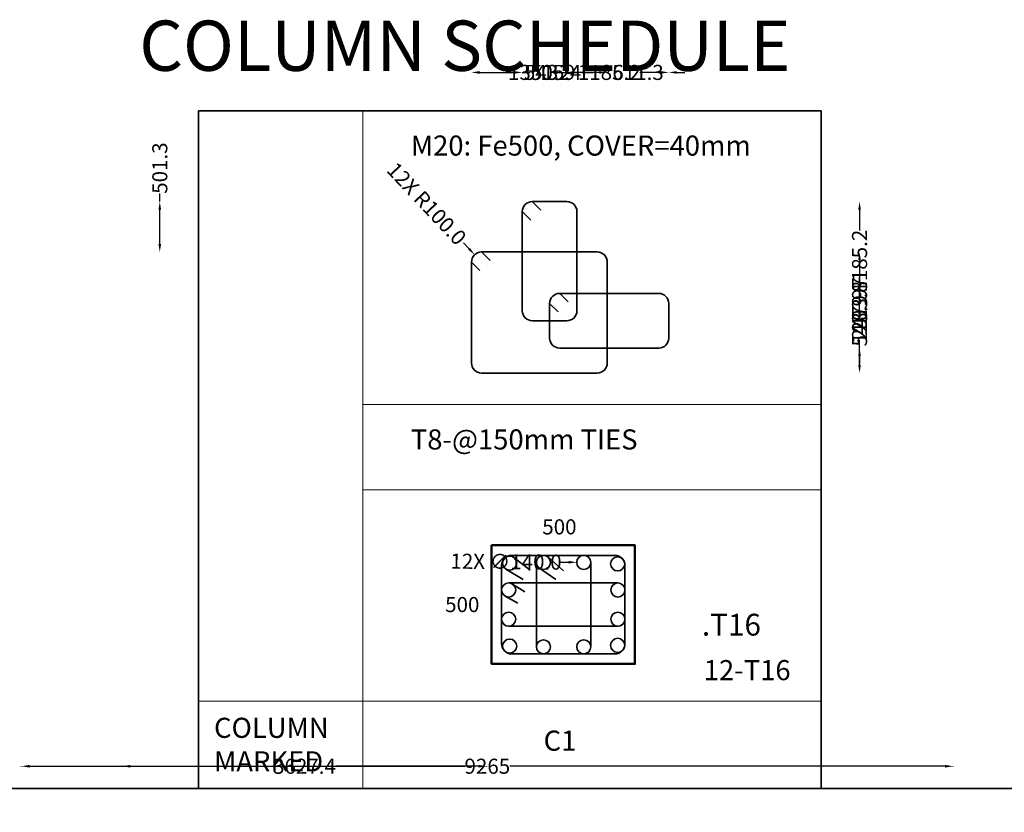
# Model space of a CAD drawing. Units: millimetres. Extents: x -19888 to 14444, y 67066 to 90098.
# Tile 6 of 7: x -7807 to 1986, y 82214 to 90098. Entities that reach past the tile are written whole.
import ezdxf

# ---------------------------------------------------------------- set-up
doc = ezdxf.new("R2010")
doc.units = ezdxf.units.MM
doc.header["$LTSCALE"] = 50
doc.header["$MEASUREMENT"] = 0
for name, color, linetype, lineweight in [('S-ANNO-DIMS', 2, 'Continuous', 18), ('S-ANNO-TABL', 7, 'Continuous', 18), ('S-ANNO-TEXT', 7, 'Continuous', 25), ('S-ANNO-TTLB', 7, 'Continuous', 35), ('S-COLS', 4, 'Continuous', 50), ('S-REIN', 6, 'Continuous', 35)]:
    doc.layers.add(name, color=color, linetype=linetype, lineweight=lineweight)
doc.styles.get("Standard").update_dxf_attribs({"font": 'arial.ttf'})
doc.dimstyles.get("Standard").update_dxf_attribs({"dimtxt": 150, "dimasz": 80, "dimexe": 0.18, "dimexo": 0.0625, "dimgap": 0.09, "dimtad": 0, "dimdec": 0, "dimzin": 0, "dimdsep": 46, "dimtxsty": 'Standard', "dimcen": 0.09, "dimadec": 0, "dimazin": 0, "dimtfac": 1, "dimtdec": 0, "dimtofl": 0, "dimtmove": 0, "dimatfit": 3, "dimfxl": 1, "dimfxlon": 1, "dimtolj": 1, "dimtzin": 0, "dimarcsym": 0})

# ---------------------------------------------------------------- blocks, each defined once
blk = doc.blocks.new('*D51')
at = {"layer": 'Defpoints', "color": 0, "ltscale": 50, "transparency": 16777216}
for p in [(1476.3, 82672.6), (-7788.5, 81596.7), (1476.3, 81596.7)]:
    blk.add_point(p, dxfattribs=at)
at = {"layer": 'S-ANNO-DIMS', "color": 0, "lineweight": -2, "ltscale": 50, "transparency": 16777216}
for p, q in [((-7788.5, 82671.6), (-7788.5, 82672.8)), ((-7708.5, 82672.6), (-3380.7, 82672.6)), ((1396.3, 82672.6), (-2931.5, 82672.6)), ((1476.3, 82671.6), (1476.3, 82672.8))]:
    blk.add_line(p, q, dxfattribs=at)
at = {"layer": 'S-ANNO-DIMS', "color": 0, "ltscale": 50, "transparency": 16777216}
for points in [[(-7708.5, 82686), (-7708.5, 82659.3), (-7788.5, 82672.6)], [(1396.3, 82686), (1396.3, 82659.3), (1476.3, 82672.6)]]:
    blk.add_solid(points, dxfattribs=at)
at = {"layer": 'S-ANNO-DIMS', "color": 0, "ltscale": 50, "transparency": 16777216, "insert": (-3156.1, 82672.6), "char_height": 150, "attachment_point": 5}
blk.add_mtext('\\A1;9265', dxfattribs=at)
blk = doc.blocks.new('*D57')
at = {"layer": 'Defpoints', "color": 0, "ltscale": 50, "transparency": 16777216}
for p in [(-3161.2, 82672.6), (-6788.5, 80274.3), (-3161.2, 80215.4)]:
    blk.add_point(p, dxfattribs=at)
at = {"layer": 'S-ANNO-DIMS', "color": 0, "lineweight": -2, "ltscale": 50, "transparency": 16777216}
for p, q in [((-6788.5, 82671.6), (-6788.5, 82672.8)), ((-6708.5, 82672.6), (-5286, 82672.6)), ((-3241.2, 82672.6), (-4663.8, 82672.6)), ((-3161.2, 82671.6), (-3161.2, 82672.8))]:
    blk.add_line(p, q, dxfattribs=at)
at = {"layer": 'S-ANNO-DIMS', "color": 0, "ltscale": 50, "transparency": 16777216}
for points in [[(-6708.5, 82686), (-6708.5, 82659.3), (-6788.5, 82672.6)], [(-3241.2, 82686), (-3241.2, 82659.3), (-3161.2, 82672.6)]]:
    blk.add_solid(points, dxfattribs=at)
at = {"layer": 'S-ANNO-DIMS', "color": 0, "ltscale": 50, "transparency": 16777216, "insert": (-4974.9, 82672.6), "char_height": 150, "attachment_point": 5}
blk.add_mtext('\\A1;3627.4', dxfattribs=at)
blk = doc.blocks.new('*D80')
at = {"layer": 'Defpoints', "color": 0, "ltscale": 50, "transparency": 16777216}
for p in [(-1962.8, 89573.9), (-3314, 86683.8), (-1962.8, 86683.8)]:
    blk.add_point(p, dxfattribs=at)
at = {"layer": 'S-ANNO-DIMS', "color": 0, "lineweight": -2, "ltscale": 50, "transparency": 16777216}
for p, q in [((-3314, 89572.9), (-3314, 89574.1)), ((-3234, 89573.9), (-2942, 89573.9)), ((-2042.8, 89573.9), (-2334.8, 89573.9)), ((-1962.8, 89572.9), (-1962.8, 89574.1))]:
    blk.add_line(p, q, dxfattribs=at)
at = {"layer": 'S-ANNO-DIMS', "color": 0, "ltscale": 50, "transparency": 16777216}
for points in [[(-3234, 89587.2), (-3234, 89560.5), (-3314, 89573.9)], [(-2042.8, 89587.2), (-2042.8, 89560.5), (-1962.8, 89573.9)]]:
    blk.add_solid(points, dxfattribs=at)
at = {"layer": 'S-ANNO-DIMS', "color": 0, "ltscale": 50, "transparency": 16777216, "insert": (-2638.4, 89573.9), "char_height": 150, "attachment_point": 5}
blk.add_mtext('\\A1;1351.2', dxfattribs=at)
blk = doc.blocks.new('*D81')
at = {"layer": 'Defpoints', "color": 0, "ltscale": 50, "transparency": 16777216}
for p in [(-2062.8, 87787.7), (-2062.8, 86583.8), (546.2, 86583.8)]:
    blk.add_point(p, dxfattribs=at)
at = {"layer": 'S-ANNO-DIMS', "color": 0, "lineweight": -2, "ltscale": 50, "transparency": 16777216}
for p, q in [((545.2, 87787.7), (546.4, 87787.7)), ((546.2, 87707.7), (546.2, 87490.3)), ((546.2, 86663.8), (546.2, 86881.2)), ((545.2, 86583.8), (546.4, 86583.8))]:
    blk.add_line(p, q, dxfattribs=at)
at = {"layer": 'S-ANNO-DIMS', "color": 0, "ltscale": 50, "transparency": 16777216}
for points in [[(532.9, 87707.7), (559.5, 87707.7), (546.2, 87787.7)], [(532.9, 86663.8), (559.5, 86663.8), (546.2, 86583.8)]]:
    blk.add_solid(points, dxfattribs=at)
at = {"layer": 'S-ANNO-DIMS', "color": 0, "ltscale": 50, "transparency": 16777216, "insert": (546.2, 87185.7), "char_height": 150, "attachment_point": 5, "rotation": 90}
blk.add_mtext('\\A1;1203.8', dxfattribs=at)
blk = doc.blocks.new('*D82')
at = {"layer": 'Defpoints', "color": 0, "ltscale": 50, "transparency": 16777216}
for p in [(-2264.7, 89573.9), (-2808.6, 88188.9), (-2264.7, 88188.9)]:
    blk.add_point(p, dxfattribs=at)
at = {"layer": 'S-ANNO-DIMS', "color": 0, "lineweight": -2, "ltscale": 50, "transparency": 16777216}
for p, q in [((-2888.6, 89573.9), (-2968.6, 89573.9)), ((-2808.6, 89572.9), (-2808.6, 89574.1)), ((-2264.7, 89572.9), (-2264.7, 89574.1)), ((-2184.7, 89573.9), (-2104.7, 89573.9))]:
    blk.add_line(p, q, dxfattribs=at)
at = {"layer": 'S-ANNO-DIMS', "color": 0, "ltscale": 50, "transparency": 16777216}
for points in [[(-2888.6, 89587.2), (-2888.6, 89560.5), (-2808.6, 89573.9)], [(-2184.7, 89587.2), (-2184.7, 89560.5), (-2264.7, 89573.9)]]:
    blk.add_solid(points, dxfattribs=at)
at = {"layer": 'S-ANNO-DIMS', "color": 0, "ltscale": 50, "transparency": 16777216, "insert": (-2536.7, 89573.9), "char_height": 150, "attachment_point": 5}
blk.add_mtext('\\A1;543.9', dxfattribs=at)
blk = doc.blocks.new('*D83')
at = {"layer": 'Defpoints', "color": 0, "ltscale": 50, "transparency": 16777216}
for p in [(-2708.6, 88288.9), (-2708.6, 87103.7), (546.2, 87103.7)]:
    blk.add_point(p, dxfattribs=at)
at = {"layer": 'S-ANNO-DIMS', "color": 0, "lineweight": -2, "ltscale": 50, "transparency": 16777216}
for p, q in [((545.2, 88288.9), (546.4, 88288.9)), ((546.2, 88208.9), (546.2, 88000)), ((546.2, 87183.7), (546.2, 87392.7)), ((545.2, 87103.7), (546.4, 87103.7))]:
    blk.add_line(p, q, dxfattribs=at)
at = {"layer": 'S-ANNO-DIMS', "color": 0, "ltscale": 50, "transparency": 16777216}
for points in [[(532.9, 88208.9), (559.5, 88208.9), (546.2, 88288.9)], [(532.9, 87183.7), (559.5, 87183.7), (546.2, 87103.7)]]:
    blk.add_solid(points, dxfattribs=at)
at = {"layer": 'S-ANNO-DIMS', "color": 0, "ltscale": 50, "transparency": 16777216, "insert": (546.2, 87696.3), "char_height": 150, "attachment_point": 5, "rotation": 90}
blk.add_mtext('\\A1;1185.2', dxfattribs=at)
blk = doc.blocks.new('*D84')
at = {"layer": 'Defpoints', "color": 0, "ltscale": 50, "transparency": 16777216}
for p in [(-1351.5, 89573.9), (-2536.7, 86931.8), (-1351.5, 86931.8)]:
    blk.add_point(p, dxfattribs=at)
at = {"layer": 'S-ANNO-DIMS', "color": 0, "lineweight": -2, "ltscale": 50, "transparency": 16777216}
for p, q in [((-2536.7, 89572.9), (-2536.7, 89574.1)), ((-2456.7, 89573.9), (-2247.7, 89573.9)), ((-1431.5, 89573.9), (-1640.5, 89573.9)), ((-1351.5, 89572.9), (-1351.5, 89574.1))]:
    blk.add_line(p, q, dxfattribs=at)
at = {"layer": 'S-ANNO-DIMS', "color": 0, "ltscale": 50, "transparency": 16777216}
for points in [[(-2456.7, 89587.2), (-2456.7, 89560.5), (-2536.7, 89573.9)], [(-1431.5, 89587.2), (-1431.5, 89560.5), (-1351.5, 89573.9)]]:
    blk.add_solid(points, dxfattribs=at)
at = {"layer": 'S-ANNO-DIMS', "color": 0, "ltscale": 50, "transparency": 16777216, "insert": (-1944.1, 89573.9), "char_height": 150, "attachment_point": 5}
blk.add_mtext('\\A1;1185.2', dxfattribs=at)
blk = doc.blocks.new('*D85')
at = {"layer": 'Defpoints', "color": 0, "ltscale": 50, "transparency": 16777216}
for p in [(-1451.5, 87375.7), (-1451.5, 86831.8), (546.2, 86831.8)]:
    blk.add_point(p, dxfattribs=at)
at = {"layer": 'S-ANNO-DIMS', "color": 0, "lineweight": -2, "ltscale": 50, "transparency": 16777216}
for p, q in [((546.2, 87455.7), (546.2, 87535.7)), ((545.2, 87375.7), (546.4, 87375.7)), ((545.2, 86831.8), (546.4, 86831.8)), ((546.2, 86751.8), (546.2, 86671.8))]:
    blk.add_line(p, q, dxfattribs=at)
at = {"layer": 'S-ANNO-DIMS', "color": 0, "ltscale": 50, "transparency": 16777216}
for points in [[(532.9, 87455.7), (559.5, 87455.7), (546.2, 87375.7)], [(532.9, 86751.8), (559.5, 86751.8), (546.2, 86831.8)]]:
    blk.add_solid(points, dxfattribs=at)
at = {"layer": 'S-ANNO-DIMS', "color": 0, "ltscale": 50, "transparency": 16777216, "insert": (546.2, 87103.7), "char_height": 150, "attachment_point": 5, "rotation": 90}
blk.add_mtext('\\A1;543.9', dxfattribs=at)
blk = doc.blocks.new('*D86')
at = {"layer": 'Defpoints', "color": 0, "ltscale": 50, "transparency": 16777216}
for p in [(-2808.6, 89573.9), (-2808.6, 88188.9), (-3314, 87687.7)]:
    blk.add_point(p, dxfattribs=at)
at = {"layer": 'S-ANNO-DIMS', "color": 0, "lineweight": -2, "ltscale": 50, "transparency": 16777216}
for p, q in [((-3314, 89572.9), (-3314, 89574.1)), ((-3234, 89573.9), (-2888.6, 89573.9)), ((-2808.6, 89572.9), (-2808.6, 89574.1)), ((-2808.6, 89573.9), (-2728.6, 89573.9))]:
    blk.add_line(p, q, dxfattribs=at)
at = {"layer": 'S-ANNO-DIMS', "color": 0, "ltscale": 50, "transparency": 16777216}
for points in [[(-3234, 89587.2), (-3234, 89560.5), (-3314, 89573.9)], [(-2888.6, 89587.2), (-2888.6, 89560.5), (-2808.6, 89573.9)]]:
    blk.add_solid(points, dxfattribs=at)
at = {"layer": 'S-ANNO-DIMS', "color": 0, "ltscale": 50, "transparency": 16777216, "insert": (-2475.8, 89573.9), "char_height": 150, "attachment_point": 5}
blk.add_mtext('\\A1;505.4', dxfattribs=at)
blk = doc.blocks.new('*D87')
at = {"layer": 'Defpoints', "color": 0, "ltscale": 50, "transparency": 16777216}
for p in [(-6414, 88288.9), (-2708.6, 88288.9), (-3214, 87787.7)]:
    blk.add_point(p, dxfattribs=at)
at = {"layer": 'S-ANNO-DIMS', "color": 0, "lineweight": -2, "ltscale": 50, "transparency": 16777216}
for p, q in [((-6414, 88288.9), (-6414, 88368.9)), ((-6413, 88288.9), (-6414.2, 88288.9)), ((-6414, 87867.7), (-6414, 88208.9)), ((-6413, 87787.7), (-6414.2, 87787.7))]:
    blk.add_line(p, q, dxfattribs=at)
at = {"layer": 'S-ANNO-DIMS', "color": 0, "ltscale": 50, "transparency": 16777216}
for points in [[(-6427.3, 88208.9), (-6400.7, 88208.9), (-6414, 88288.9)], [(-6427.3, 87867.7), (-6400.7, 87867.7), (-6414, 87787.7)]]:
    blk.add_solid(points, dxfattribs=at)
at = {"layer": 'S-ANNO-DIMS', "color": 0, "ltscale": 50, "transparency": 16777216, "insert": (-6414, 88622.1), "char_height": 150, "attachment_point": 5, "rotation": 90}
blk.add_mtext('\\A1;501.3', dxfattribs=at)
blk = doc.blocks.new('*D88')
at = {"layer": 'Defpoints', "color": 0, "ltscale": 50, "transparency": 16777216}
for p in [(-1351.5, 89573.9), (-1351.5, 86931.8), (-1962.8, 86683.8)]:
    blk.add_point(p, dxfattribs=at)
at = {"layer": 'S-ANNO-DIMS', "color": 0, "lineweight": -2, "ltscale": 50, "transparency": 16777216}
for p, q in [((-2042.8, 89573.9), (-2122.8, 89573.9)), ((-1962.8, 89572.9), (-1962.8, 89574.1)), ((-1351.5, 89572.9), (-1351.5, 89574.1)), ((-1271.5, 89573.9), (-1191.5, 89573.9))]:
    blk.add_line(p, q, dxfattribs=at)
at = {"layer": 'S-ANNO-DIMS', "color": 0, "ltscale": 50, "transparency": 16777216}
for points in [[(-2042.8, 89587.2), (-2042.8, 89560.5), (-1962.8, 89573.9)], [(-1271.5, 89587.2), (-1271.5, 89560.5), (-1351.5, 89573.9)]]:
    blk.add_solid(points, dxfattribs=at)
at = {"layer": 'S-ANNO-DIMS', "color": 0, "ltscale": 50, "transparency": 16777216, "insert": (-1657.2, 89573.9), "char_height": 150, "attachment_point": 5}
blk.add_mtext('\\A1;611.3', dxfattribs=at)
blk = doc.blocks.new('*D89')
at = {"layer": 'Defpoints', "color": 0, "ltscale": 50, "transparency": 16777216}
for p in [(-2436.7, 86831.8), (546.2, 86831.8), (-2062.8, 86583.8)]:
    blk.add_point(p, dxfattribs=at)
at = {"layer": 'S-ANNO-DIMS', "color": 0, "lineweight": -2, "ltscale": 50, "transparency": 16777216}
for p, q in [((546.2, 86831.8), (546.2, 86911.8)), ((545.2, 86831.8), (546.4, 86831.8)), ((546.2, 86663.8), (546.2, 86751.8)), ((545.2, 86583.8), (546.4, 86583.8))]:
    blk.add_line(p, q, dxfattribs=at)
at = {"layer": 'S-ANNO-DIMS', "color": 0, "ltscale": 50, "transparency": 16777216}
for points in [[(532.9, 86751.8), (559.5, 86751.8), (546.2, 86831.8)], [(532.9, 86663.8), (559.5, 86663.8), (546.2, 86583.8)]]:
    blk.add_solid(points, dxfattribs=at)
at = {"layer": 'S-ANNO-DIMS', "color": 0, "ltscale": 50, "transparency": 16777216, "insert": (546.2, 87224.5), "char_height": 150, "attachment_point": 5, "rotation": 90}
blk.add_mtext('\\A1;247.97', dxfattribs=at)
blk = doc.blocks.new('*D100')
at = {"layer": 'Defpoints', "color": 0, "ltscale": 50, "transparency": 16777216}
for p in [(-3282.5, 87760.6), (-3214, 87687.7)]:
    blk.add_point(p, dxfattribs=at)
at = {"layer": 'S-ANNO-DIMS', "color": 0, "lineweight": -2, "ltscale": 50, "transparency": 16777216}
for p, q in [((-3392, 87877.2), (-3337.2, 87818.9)), ((-3214.1, 87687.7), (-3213.9, 87687.7)), ((-3214, 87687.6), (-3214, 87687.8))]:
    blk.add_line(p, q, dxfattribs=at)
at = {"layer": 'S-ANNO-DIMS', "color": 0, "ltscale": 50, "transparency": 16777216}
blk.add_solid([(-3327.5, 87828), (-3346.9, 87809.7), (-3282.5, 87760.6)], dxfattribs=at)
at = {"layer": 'S-ANNO-DIMS', "color": 0, "ltscale": 50, "transparency": 16777216, "insert": (-3759.7, 88268.7), "char_height": 150, "attachment_point": 5, "rotation": 313.20425}
blk.add_mtext('\\A1;12X R100.0', dxfattribs=at)
blk = doc.blocks.new('*D101')
at = {"layer": 'Defpoints', "color": 0, "ltscale": 50, "transparency": 16777216}
for p in [(-2267.3, 84701), (-2127.3, 84699.7)]:
    blk.add_point(p, dxfattribs=at)
at = {"layer": 'S-ANNO-DIMS', "color": 0, "lineweight": -2, "ltscale": 50, "transparency": 16777216}
for p, q in [((-2427.3, 84702.5), (-2347.3, 84701.8)), ((-2197.4, 84700.3), (-2197.2, 84700.3)), ((-2197.3, 84700.2), (-2197.3, 84700.4))]:
    blk.add_line(p, q, dxfattribs=at)
at = {"layer": 'S-ANNO-DIMS', "color": 0, "ltscale": 50, "transparency": 16777216}
blk.add_solid([(-2347.2, 84715.1), (-2347.4, 84688.4), (-2267.3, 84701)], dxfattribs=at)
at = {"layer": 'S-ANNO-DIMS', "color": 0, "ltscale": 50, "transparency": 16777216, "insert": (-2970.2, 84707.7), "char_height": 150, "attachment_point": 5, "rotation": 359.45387}
blk.add_mtext('\\A1;12X ∅140.0', dxfattribs=at)

msp = doc.modelspace()

# ---------------------------------------------------------------- linework, layer by layer
at = {"layer": 'S-ANNO-TABL', "ltscale": 50}
for p, q in [((-4395.763, 89190.426), (-4395.763, 82452.304)), ((-4395.763, 86270.369), (162.755, 86270.369)), ((-4395.763, 85422.611), (162.755, 85422.611)), ((-6030.541, 83318.914), (162.755, 83318.914))]:
    msp.add_line(p, q, dxfattribs=at)
at = {"layer": 'S-ANNO-TTLB', "ltscale": 50}
for points in [[(-6030.541, 89190.426), (162.755, 89190.426), (162.755, 82452.304), (-6030.541, 82452.304)], [(-8639.597, 82452.304), (5654.103, 82452.304), (5654.103, 77078.62), (-8639.597, 77078.62)]]:
    msp.add_lwpolyline(points, close=True, dxfattribs=at)
at = {"layer": 'S-COLS', "ltscale": 50}
msp.add_lwpolyline([(-3113.905, 84870.336), (-1687.616, 84870.336), (-1687.616, 83690.282), (-3113.905, 83690.282)], close=True, dxfattribs=at)
at = {"layer": 'S-REIN', "ltscale": 50}
for p, q in [((-2708.626, 88288.92), (-2623.773, 88204.067)), ((-2808.626, 88188.92), (-2723.773, 88104.067)), ((-3214.001, 87787.664), (-3129.148, 87702.811)), ((-3314.001, 87687.664), (-3229.148, 87602.811)), ((-2436.681, 87375.689), (-2351.828, 87290.836)), ((-2536.681, 87275.689), (-2451.828, 87190.836)), ((-2891.17, 84748.25), (-2728.533, 84622.929)), ((-2551.529, 84752.569), (-2397.79, 84615.404)), ((-2970.555, 84633.169), (-2800.973, 84528.92)), ((-2668.131, 84700.336), (-2668.131, 83860.282)), ((-2647.436, 84650.647), (-2474.201, 84529.76)), ((-2127.312, 84700.336), (-2127.312, 83860.282)), ((-1857.616, 84495.714), (-2943.905, 84495.714)), ((-2906.794, 84485.068), (-2783.391, 84407.91)), ((-2977.705, 84364.415), (-2853.43, 84295.892)), ((-1857.616, 84064.903), (-2943.905, 84064.903))]:
    msp.add_line(p, q, dxfattribs=at)
for points in [[(-2708.626, 88288.92), (-2364.736, 88288.92, -0.41421356), (-2264.736, 88188.92), (-2264.736, 87203.744, -0.41421356), (-2364.736, 87103.744), (-2708.626, 87103.744, -0.41421356), (-2808.626, 87203.744), (-2808.626, 88188.92, -0.41421356)], [(-3214.001, 87787.664), (-2062.841, 87787.664, -0.41421356), (-1962.841, 87687.664), (-1962.841, 86683.83, -0.41421356), (-2062.841, 86583.83), (-3214.001, 86583.83, -0.41421356), (-3314.001, 86683.83), (-3314.001, 87687.664, -0.41421356)], [(-1351.505, 87275.689), (-1351.505, 86931.798, -0.41421356), (-1451.505, 86831.798), (-2436.681, 86831.798, -0.41421356), (-2536.681, 86931.798), (-2536.681, 87275.689, -0.41421356), (-2436.681, 87375.689), (-1451.505, 87375.689, -0.41421356)], [(-2913.905, 84770.336), (-1887.616, 84770.336, -0.41421356), (-1787.616, 84670.336), (-1787.616, 83890.282, -0.41421356), (-1887.616, 83790.282), (-2913.905, 83790.282, -0.41421356), (-3013.905, 83890.282), (-3013.905, 84670.336, -0.41421356)]]:
    msp.add_lwpolyline(points, format="xyb", close=True, dxfattribs=at)
for centre in [(-2933.896, 84692.802), (-2598.131, 84700.336), (-2197.312, 84700.336), (-1859.767, 84685.703), (-2943.905, 84425.714), (-1857.616, 84425.714), (-2943.905, 84134.903), (-1857.616, 84134.903), (-2933.896, 83867.815), (-2598.131, 83860.282), (-2197.312, 83860.282), (-1859.767, 83874.914)]:
    msp.add_circle(centre, 70, dxfattribs=at)

# ---------------------------------------------------------------- texts
at = {"layer": 'S-ANNO-TEXT', "ltscale": 50, "attachment_point": 1}
for s, width, insert, char_height in [('COLUMN SCHEDULE', 7482.5403, (-6618.001, 90089.361), 500), ('M20: Fe500, COVER=40mm', 3937.67384, (-3917.027, 88946.235), 200), ('T8-@150mm TIES', 3937.67384, (-3917.027, 86023.179), 200), ('500', 1609.35955, (-2609.818, 85128.734), 150), ('500', 1609.35955, (-3575.772, 84355.782), 150), ('{\\H1.08333x;.T16}', 1609.35955, (-1022.1, 84189.039), 200), ('12-T16', 1609.35955, (-1003.66, 83728.649), 200), ('COLUMN\\PMARKED', 1609.35955, (-5874.459, 83154.851), 200), ('C1', 1609.35955, (-2596.41, 83027.099), 200)]:
    msp.add_mtext_dynamic_manual_height_columns(s, width=width, gutter_width=1, heights=[0], dxfattribs=dict(at, insert=insert, char_height=char_height))

# ---------------------------------------------------------------- dimensions: what is measured, and where the dimension line sits
at = {"layer": 'S-ANNO-DIMS', "ltscale": 50}
for base, p1, p2, override, picture, middle in [((-1962.841, 89573.876), (-3314.001, 86683.83), (-1962.841, 86683.83), {"dimdec": 1, "dimlfac": 1, "dimrnd": 0, "dimzin": 0, "dimdsep": 46, "dimlunit": 2}, '*D80', (-2638.421, 89573.876)), ((-2808.626, 89573.876), (-3314.001, 87687.664), (-2808.626, 88188.92), {"dimdec": 1, "dimlfac": 1, "dimrnd": 0, "dimzin": 0, "dimdsep": 46, "dimlunit": 2}, '*D86', (-2475.756, 89573.876)), ((-2264.736, 89573.876), (-2808.626, 88188.92), (-2264.736, 88188.92), {"dimdec": 1, "dimlfac": 1, "dimrnd": 0, "dimzin": 0, "dimdsep": 46, "dimlunit": 2}, '*D82', (-2536.681, 89573.876)), ((-1351.505, 89573.876), (-2536.681, 86931.798), (-1351.505, 86931.798), {"dimdec": 1, "dimlfac": 1, "dimrnd": 0, "dimzin": 0, "dimdsep": 46, "dimlunit": 2}, '*D84', (-1944.093, 89573.876)), ((-1351.505, 89573.876), (-1962.841, 86683.83), (-1351.505, 86931.798), {"dimdec": 1, "dimlfac": 1, "dimrnd": 0, "dimzin": 0, "dimdsep": 46, "dimlunit": 2}, '*D88', (-1657.173, 89573.876)), ((1476.348, 82672.634), (-7788.546, 81596.699), (1476.348, 81596.699), {"dimdec": 0, "dimlfac": 1, "dimrnd": 0, "dimzin": 0, "dimdsep": 46, "dimlunit": 2}, '*D51', (-3156.099, 82672.634)), ((-3161.177, 82672.634), (-6788.546, 80274.282), (-3161.177, 80215.359), {"dimdec": 1, "dimlfac": 1, "dimrnd": 0, "dimzin": 0, "dimdsep": 46, "dimlunit": 2}, '*D57', (-4974.862, 82672.634))]:
    dim = msp.add_linear_dim(base=base, p1=p1, p2=p2, dimstyle='Standard', override=override, dxfattribs=at)
    dim.commit()
    dim.dimension.update_dxf_attribs({"geometry": picture, "text_midpoint": middle})
for base, p1, p2, override, picture, middle in [((-6413.991, 88288.92), (-3214.001, 87787.664), (-2708.626, 88288.92), {"dimdec": 1, "dimlfac": 1, "dimrnd": 0, "dimzin": 0, "dimdsep": 46, "dimlunit": 2}, '*D87', (-6413.991, 88622.096)), ((546.205, 87103.744), (-2708.626, 88288.92), (-2708.626, 87103.744), {"dimdec": 1, "dimlfac": 1, "dimrnd": 0, "dimzin": 0, "dimdsep": 46, "dimlunit": 2}, '*D83', (546.205, 87696.332)), ((546.205, 86583.83), (-2062.841, 87787.664), (-2062.841, 86583.83), {"dimdec": 1, "dimlfac": 1, "dimrnd": 0, "dimzin": 0, "dimdsep": 46, "dimlunit": 2}, '*D81', (546.205, 87185.747)), ((546.205, 86831.798), (-2062.841, 86583.83), (-2436.681, 86831.798), {"dimdec": 2, "dimlfac": 1, "dimrnd": 0, "dimzin": 0, "dimdsep": 46, "dimlunit": 2}, '*D89', (546.205, 87224.525)), ((546.205, 86831.798), (-1451.505, 87375.689), (-1451.505, 86831.798), {"dimdec": 1, "dimlfac": 1, "dimrnd": 0, "dimzin": 0, "dimdsep": 46, "dimlunit": 2}, '*D85', (546.205, 87103.744))]:
    dim = msp.add_linear_dim(base=base, p1=p1, p2=p2, angle=90, dimstyle='Standard', override=override, dxfattribs=at)
    dim.commit()
    dim.dimension.update_dxf_attribs({"geometry": picture, "text_midpoint": middle})
dim = msp.add_radius_dim(center=(-3214.001, 87687.664), mpoint=(-3282.461, 87760.556), text='12X <>', dimstyle='Standard', override={"dimdec": 1, "dimlfac": 1, "dimrnd": 0, "dimzin": 0, "dimdsep": 46, "dimlunit": 2}, dxfattribs=at)
dim.commit()
dim.dimension.update_dxf_attribs({"geometry": '*D100', "text_midpoint": (-3759.67, 88268.656)})
dim = msp.add_diameter_dim_2p(p1=(-2127.315, 84699.669), p2=(-2267.308, 84701.003), text='12X <>', dimstyle='Standard', override={"dimdec": 1, "dimlfac": 1, "dimrnd": 0, "dimzin": 0, "dimdsep": 46, "dimlunit": 2}, dxfattribs=at)
dim.commit()
dim.dimension.update_dxf_attribs({"geometry": '*D101', "text_midpoint": (-2970.17, 84707.703)})

doc.saveas('drawing.dxf')
